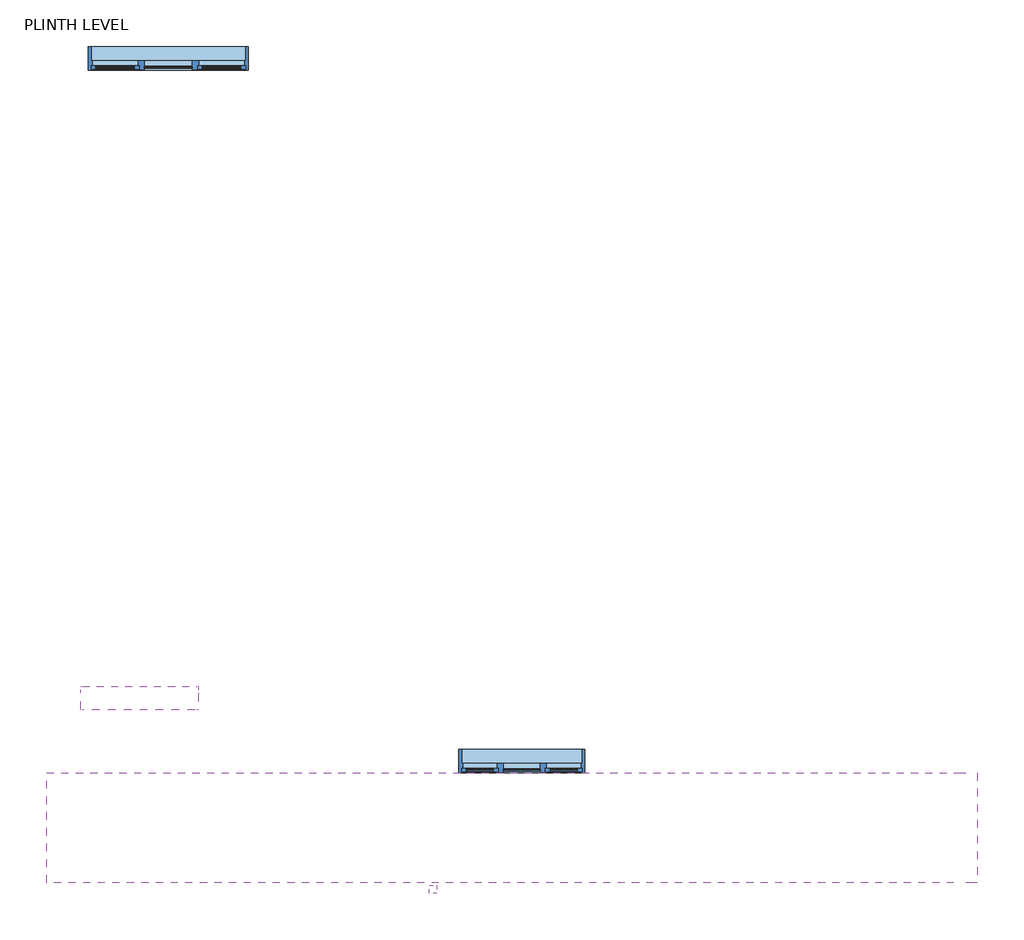
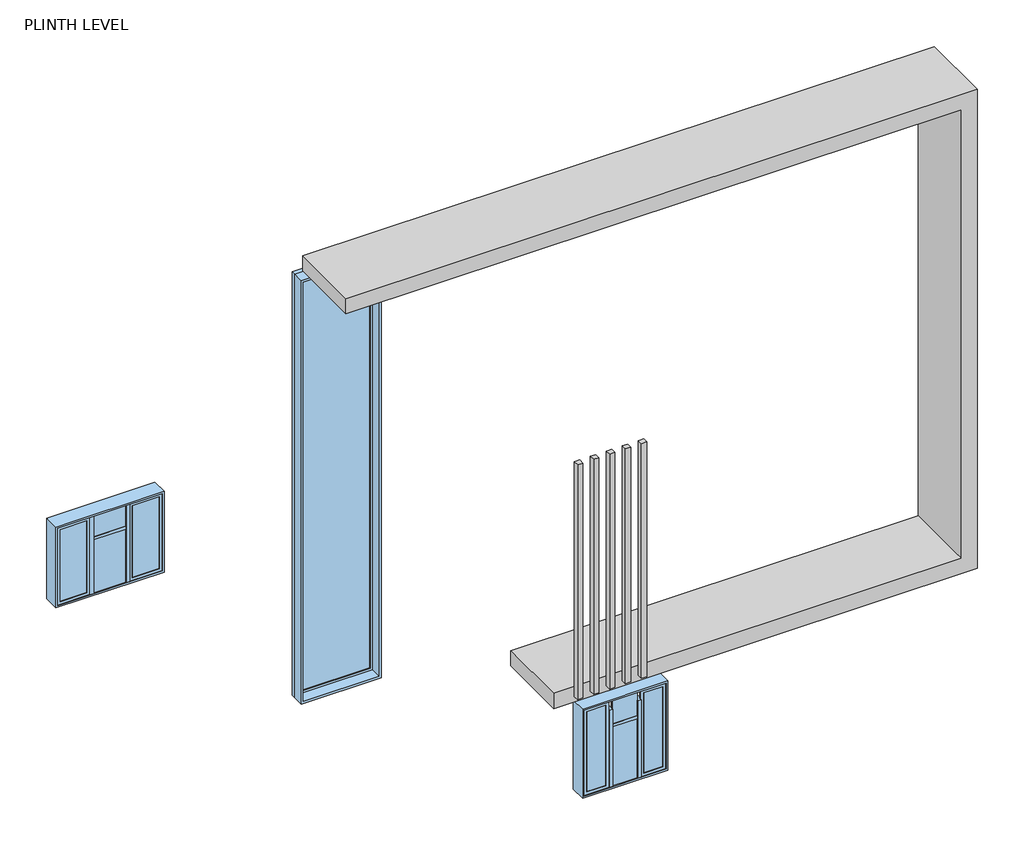
# One storey: 3 windows, 2 proxies.
"""IFC4 building model written with IfcOpenShell, lengths in millimetres."""

from ifc_helpers import new_model, si_unit, origin, place, context, project, spatial, transform, mapped, element, save
from components import generic_models_3_generic_models_3_22da3405, generic_models_7_generic_models_7_f5532255, fixed_21_x3_9_7c61b802, window_273a115f, window_8c4be023

model = new_model("IFC4")

# Units and contexts
model_context = context("Model", 3, world=origin())
ifc_project = project(units=[si_unit("LENGTHUNIT", "METRE", prefix="MILLI")], contexts=[model_context])

# Site, building, storey
site = spatial("IfcSite", under=ifc_project)
building = spatial("IfcBuilding", under=site)
storey = spatial("IfcBuildingStorey", under=building, Name="PLINTH LEVEL", Elevation=914.4)

# Proxies
placement = place(None, origin())
generic_models_3_generic_models_3_shape = generic_models_3_generic_models_3_22da3405(model_context)
element("IfcBuildingElementProxy", 1, Name="Generic Models 3 : Generic Models 3", ObjectType="Generic Models 3 : Generic Models 3", at=placement, inside=storey, context=model_context, shape_type="MappedRepresentation", body=[
    mapped(generic_models_3_generic_models_3_shape, transform((0.0, 0.0, 0.0), x_axis=(1.0, 0.0, 0.0), y_axis=(0.0, 1.0, 0.0), z_axis=(0.0, 0.0, 1.0))),
])
generic_models_7_generic_models_7_shape = generic_models_7_generic_models_7_f5532255(model_context)
element("IfcBuildingElementProxy", 2, Name="Generic Models 7 : Generic Models 7", ObjectType="Generic Models 7 : Generic Models 7", at=placement, inside=storey, context=model_context, shape_type="MappedRepresentation", body=[
    mapped(generic_models_7_generic_models_7_shape, transform((0.0, 0.0, 0.0), x_axis=(1.0, 0.0, 0.0), y_axis=(0.0, 1.0, 0.0), z_axis=(0.0, 0.0, 1.0))),
])

# Windows
fixed_21_x3_9_shape = fixed_21_x3_9_7c61b802(model_context)
element("IfcWindow", 3, ObjectType="Fixed : 21'x3'9'", at=placement, inside=storey, context=model_context, shape_type="MappedRepresentation", body=[
    mapped(fixed_21_x3_9_shape, transform((1086.9271331, -11251.8643494, 3022.6), x_axis=(1.0, 0.0, 0.0), y_axis=(0.0, 1.0, 0.0), z_axis=(0.0, 0.0, 1.0))),
])
window_shape = window_273a115f(model_context)
element("IfcWindow", 4, ObjectType="Window-Casement-Triple-Middle-Transom : 48\" x 53\"", at=placement, inside=storey, context=model_context, shape_type="MappedRepresentation", body=[
    mapped(window_shape, transform((4757.2271331, -11861.4643494, 914.4), x_axis=(-1.0, 0.0, 0.0), y_axis=(0.0, -1.0, 0.0), z_axis=(0.0, 0.0, 1.0))),
])
window_2_shape = window_8c4be023(model_context)
element("IfcWindow", 5, ObjectType="Window-Casement-Triple-Middle-Transom : 61\" x 48\"", at=placement, inside=storey, context=model_context, shape_type="MappedRepresentation", body=[
    mapped(window_2_shape, transform((1328.2271331, -5041.5643494, 914.4), x_axis=(-1.0, 0.0, 0.0), y_axis=(0.0, -1.0, 0.0), z_axis=(0.0, 0.0, 1.0))),
])

save(model, "model.ifc")

# Revit data of these elements
# Type "Fixed : 21'x3'9'"
#   Type Mark = "21"
#   Construction Type Id = "GSP4R"
#   Assembly Code = "B2020100"
#   Analytic Construction = "1/8 in Pilkington single glazing"
#   Visual Light Transmittance = 0.9
#   Solar Heat Gain Coefficient = 0.78
#   Heat Transfer Coefficient (U) = 0.6496 BTU/(h·ft²·°F)
#   Height = 21' - 0"
#   Default Sill Height = 3' - 9"
#   Width = 3' - 9"
#   Window Inset = 0' - 0 3/4"
#   Define Thermal Properties by = 1
#   Glass Pane Material = Glass
#   Sash Material = Sash
#   Wall Closure = (empty or 0)
# Type "Window-Casement-Triple-Middle-Transom : 48\" x 53\""
#   Type Mark = "18"
#   Fire Rating = "0.5h"
#   Assembly Code = "B2020100"
#   Analytic Construction = "Double glazing - domestic"
#   Window Width = 1' - 4"
#   Window Inset [instance default] = 0' - 0 5/8"
#   Wall Thickness [instance default] = 0' - 6"
#   Visual Light Transmittance = 0.81
#   Transom Height Ratio = 0.3
#   Thermal Resistance (R) = 1.8146 (h·ft²·°F)/BTU
#   Solar Heat Gain Coefficient = 0.76
#   Rough Width = 4' - 0 1/2"
#   Rough Height = 4' - 5 1/2"
#   Heat Transfer Coefficient (U) = 0.5511 BTU/(h·ft²·°F)
#   Height = 4' - 5"
#   Transom Height = 1' - 3.9"
#   Frame Gap 3 [instance default] = 0' - 1 83/128"
#   Frame Gap 2 [instance default] = 0' - 0 5/8"
#   Frame Gap 1 = 0' - 1 51/128"
#   Default Sill Height = 3' - 0"
#   Width = 4' - 0"
#   Frame Material = Metal - Aluminum
#   Glass Panel Material = Glass
#   Wall Closure = (empty or 0)
# Type "Window-Casement-Triple-Middle-Transom : 61\" x 48\""
#   Type Mark = "19"
#   Fire Rating = "0.5h"
#   Assembly Code = "B2020100"
#   Analytic Construction = "Double glazing - domestic"
#   Window Width = 1' - 8.33333"
#   Window Inset [instance default] = 0' - 0 5/8"
#   Wall Thickness [instance default] = 0' - 6"
#   Visual Light Transmittance = 0.81
#   Transom Height Ratio = 0.3
#   Thermal Resistance (R) = 1.8146 (h·ft²·°F)/BTU
#   Solar Heat Gain Coefficient = 0.76
#   Rough Width = 5' - 1 1/2"
#   Rough Height = 4' - 0 1/2"
#   Heat Transfer Coefficient (U) = 0.5511 BTU/(h·ft²·°F)
#   Height = 4' - 0"
#   Transom Height = 1' - 2.4"
#   Frame Gap 3 [instance default] = 0' - 1 83/128"
#   Frame Gap 2 [instance default] = 0' - 0 5/8"
#   Frame Gap 1 = 0' - 1 51/128"
#   Default Sill Height = 3' - 0"
#   Width = 5' - 1"
#   Frame Material = Metal - Aluminum
#   Glass Panel Material = Glass
#   Wall Closure = (empty or 0)
# Element 1 (IfcBuildingElementProxy, "Generic Models 3 : Generic Models 3")
#   Phase Created = New Construction
# Element 2 (IfcBuildingElementProxy, "Generic Models 7 : Generic Models 7")
#   Phase Created = New Construction
# Element 3 (IfcWindow, "Fixed : 21'x3'9'")
#   Mark = "10"
#   Phase Created = New Construction
#   Materials on its faces: "Sash", "Glass"
# Element 4 (IfcWindow, "Window-Casement-Triple-Middle-Transom : 48\" x 53\"")
#   Mark = "1"
#   Window Inset = 0' - 0 5/8"
#   Frame Gap 3 = 0' - 1 83/128"
#   Frame Gap 2 = 0' - 0 5/8"
#   Phase Created = New Construction
#   Materials on its faces: "Metal - Aluminum", "Glass"
# Element 5 (IfcWindow, "Window-Casement-Triple-Middle-Transom : 61\" x 48\"")
#   Mark = "2"
#   Window Inset = 0' - 0 5/8"
#   Frame Gap 3 = 0' - 1 83/128"
#   Frame Gap 2 = 0' - 0 5/8"
#   Phase Created = New Construction
#   Materials on its faces: "Metal - Aluminum", "Glass"
# Materials
#   "Glass": class "Glass", colour RGB 0 128 192, transparency 0.75, Description = "Soda Lime Glass", Cost = 0
#   "Sash": class "Wood", colour RGB 224 178 126, transparency 0, Cost = 0
#   "Metal - Aluminum": class "Metal", colour RGB 247 247 247, transparency 0
